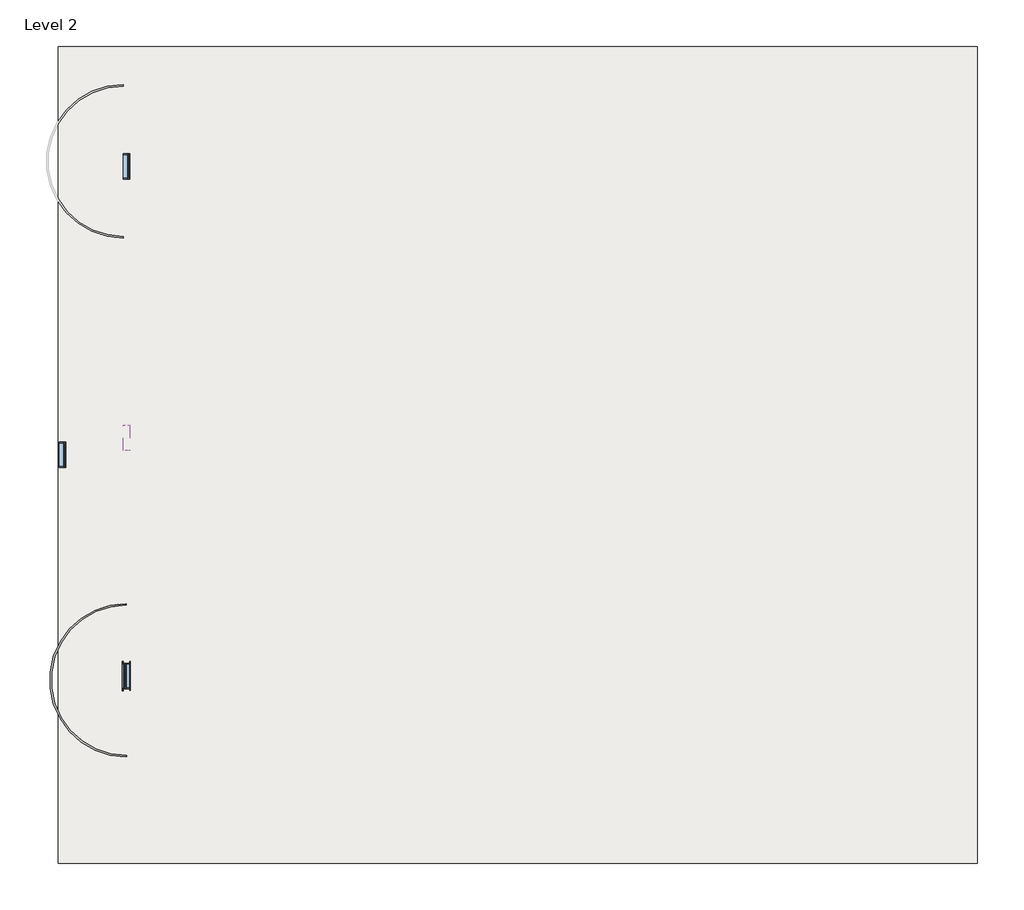
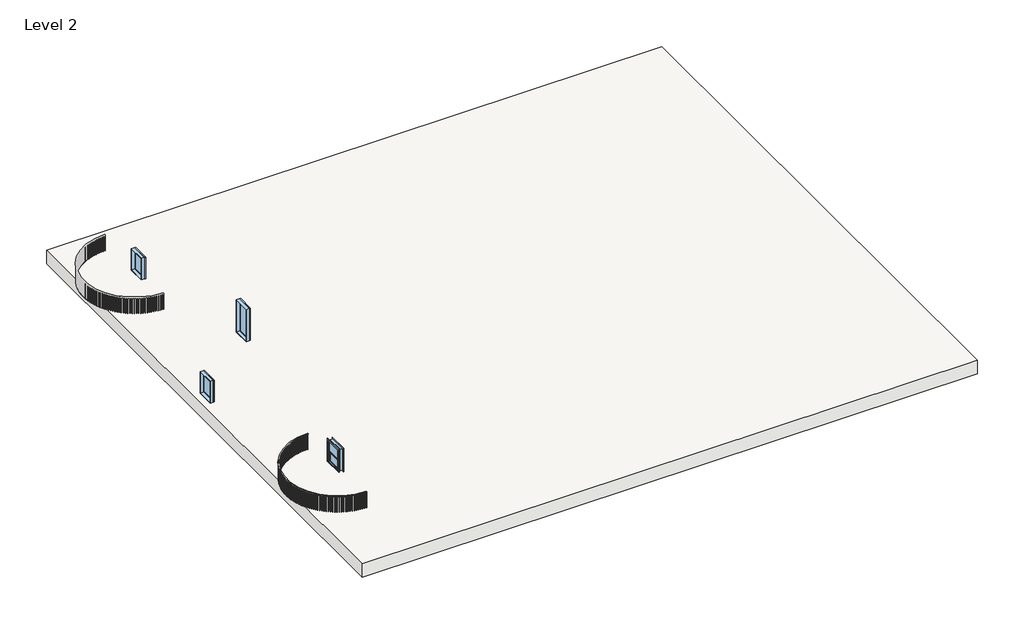
# One storey, part 1 of 2: 4 windows, 1 railing, 1 slab.
"""IFC4 building model written with IfcOpenShell, lengths in millimetres."""

from ifc_helpers import new_model, si_unit, point, frame, frame_2d, origin, place, context, project, spatial, polyline, circle_curve, trimmed, segment, composite_curve, outline, extrude, transform, mapped, element, save
from components import window_f24a59ae, window_c1f32544, window_c796fc87

model = new_model("IFC4")

# Units and contexts
model_context = context("Model", 3, world=origin())
ifc_project = project(units=[si_unit("LENGTHUNIT", "METRE", prefix="MILLI")], contexts=[model_context])

# Site, building, storey
site = spatial("IfcSite", under=ifc_project)
building = spatial("IfcBuilding", under=site)
storey = spatial("IfcBuildingStorey", under=building, Name="Level 2", Elevation=3048.0)

# Railing
placement = place(None, origin())
element("IfcRailing", 1, ObjectType="Handrail - Rectangular", at=placement, inside=storey, context=model_context, shape_type="SweptSolid", body=[
    extrude(outline(composite_curve([segment(trimmed(circle_curve(frame_2d((-15613.8723021, -8267.0443987)), 2743.2), [point((-15613.8723021, -11010.2443987))], [point((-15613.8723021, -5523.8443987))], False, "CARTESIAN"), True, "CONTINUOUS"), segment(polyline([(-15613.8723021, -5523.8443987), (-15613.8723021, -5574.6443987)]), True, "CONTINUOUS"), segment(trimmed(circle_curve(frame_2d((-15613.8723021, -8267.0443987)), 2692.4), [point((-15613.8723021, -5574.6443987))], [point((-15613.8723021, -10959.4443987))], True, "CARTESIAN"), True, "CONTINUOUS"), segment(polyline([(-15613.8723021, -10959.4443987), (-15613.8723021, -11010.2443987)]), True, "CONTINUOUS")], self_intersect=False)), frame((0.0, 0.0, 3911.6), z_axis=(0.0, 0.0, 1.0), x_axis=(1.0, 0.0, 0.0)), (0.0, 0.0, 1.0), 50.8),
    extrude(outline(polyline([(-15627.231195, -10994.3533143), (-15627.2044157, -10975.3033331), (-15608.1544345, -10975.3301124), (-15608.1812138, -10994.3800936), (-15627.231195, -10994.3533143)])), frame((0.0, 0.0, 3048.0), z_axis=(0.0, 0.0, 1.0), x_axis=(1.0, 0.0, 0.0)), (0.0, 0.0, 1.0), 863.6),
    extrude(outline(polyline([(-15729.1535895, -10991.9485449), (-15728.414846, -10972.9128742), (-15709.3791753, -10973.6516178), (-15710.1179188, -10992.6872885), (-15729.1535895, -10991.9485449)])), frame((0.0, 0.0, 3048.0), z_axis=(0.0, 0.0, 1.0), x_axis=(1.0, 0.0, 0.0)), (0.0, 0.0, 1.0), 863.6),
    extrude(outline(polyline([(-15830.914897, -10985.7361601), (-15829.4652214, -10966.7413992), (-15810.4704606, -10968.1910747), (-15811.9201361, -10987.1858356), (-15830.914897, -10985.7361601)])), frame((0.0, 0.0, 3048.0), z_axis=(0.0, 0.0, 1.0), x_axis=(1.0, 0.0, 0.0)), (0.0, 0.0, 1.0), 863.6),
    extrude(outline(polyline([(-15932.3729223, -10975.7248406), (-15930.2143405, -10956.7975316), (-15911.2870315, -10958.9561134), (-15913.4456133, -10977.8834224), (-15932.3729223, -10975.7248406)])), frame((0.0, 0.0, 3048.0), z_axis=(0.0, 0.0, 1.0), x_axis=(1.0, 0.0, 0.0)), (0.0, 0.0, 1.0), 863.6),
    extrude(outline(polyline([(-16033.3858942, -10961.9285757), (-16030.5214224, -10943.0951665), (-16011.6880132, -10945.9596384), (-16014.5524851, -10964.7930475), (-16033.3858942, -10961.9285757)])), frame((0.0, 0.0, 3048.0), z_axis=(0.0, 0.0, 1.0), x_axis=(1.0, 0.0, 0.0)), (0.0, 0.0, 1.0), 863.6),
    extrude(outline(polyline([(-16133.8126634, -10944.3666434), (-16130.2463041, -10925.6534507), (-16111.5331114, -10929.2198099), (-16115.0994706, -10947.9330026), (-16133.8126634, -10944.3666434)])), frame((0.0, 0.0, 3048.0), z_axis=(0.0, 0.0, 1.0), x_axis=(1.0, 0.0, 0.0)), (0.0, 0.0, 1.0), 863.6),
    extrude(outline(polyline([(-16233.5128994, -10923.0635838), (-16229.2496362, -10904.4967562), (-16210.6828086, -10908.7600194), (-16214.9460718, -10927.326847), (-16233.5128994, -10923.0635838)])), frame((0.0, 0.0, 3048.0), z_axis=(0.0, 0.0, 1.0), x_axis=(1.0, 0.0, 0.0)), (0.0, 0.0, 1.0), 863.6),
    extrude(outline(polyline([(-16332.3472874, -10898.0491643), (-16327.3930774, -10879.654646), (-16308.9985591, -10884.608856), (-16313.9527691, -10903.0033743), (-16332.3472874, -10898.0491643)])), frame((0.0, 0.0, 3048.0), z_axis=(0.0, 0.0, 1.0), x_axis=(1.0, 0.0, 0.0)), (0.0, 0.0, 1.0), 863.6),
    extrude(outline(polyline([(-16430.1777221, -10869.3583388), (-16424.5394881, -10851.1618331), (-16406.3429824, -10856.8000671), (-16411.9812164, -10874.9965728), (-16430.1777221, -10869.3583388)])), frame((0.0, 0.0, 3048.0), z_axis=(0.0, 0.0, 1.0), x_axis=(1.0, 0.0, 0.0)), (0.0, 0.0, 1.0), 863.6),
    extrude(outline(polyline([(-16526.8675012, -10837.0311978), (-16520.5531216, -10819.0581316), (-16502.5800554, -10825.3725111), (-16508.8944349, -10843.3455773), (-16526.8675012, -10837.0311978)])), frame((0.0, 0.0, 3048.0), z_axis=(0.0, 0.0, 1.0), x_axis=(1.0, 0.0, 0.0)), (0.0, 0.0, 1.0), 863.6),
    extrude(outline(polyline([(-16622.2815163, -10801.1129136), (-16615.2998146, -10783.3884011), (-16597.5753021, -10790.3701028), (-16604.5570038, -10808.0946153), (-16622.2815163, -10801.1129136)])), frame((0.0, 0.0, 3048.0), z_axis=(0.0, 0.0, 1.0), x_axis=(1.0, 0.0, 0.0)), (0.0, 0.0, 1.0), 863.6),
    extrude(outline(polyline([(-16716.2864416, -10761.653676), (-16708.6471735, -10744.2024845), (-16691.1959821, -10751.8417526), (-16698.8352501, -10769.292944), (-16716.2864416, -10761.653676)])), frame((0.0, 0.0, 3048.0), z_axis=(0.0, 0.0, 1.0), x_axis=(1.0, 0.0, 0.0)), (0.0, 0.0, 1.0), 863.6),
    extrude(outline(polyline([(-16808.7509204, -10718.708623), (-16800.4647607, -10701.5551378), (-16783.3112754, -10709.8412975), (-16791.5974352, -10726.9947828), (-16808.7509204, -10718.708623)])), frame((0.0, 0.0, 3048.0), z_axis=(0.0, 0.0, 1.0), x_axis=(1.0, 0.0, 0.0)), (0.0, 0.0, 1.0), 863.6),
    extrude(outline(polyline([(-16899.5457485, -10672.3377634), (-16890.6242756, -10655.5059536), (-16873.7924658, -10664.4274266), (-16882.7139387, -10681.2592364), (-16899.5457485, -10672.3377634)])), frame((0.0, 0.0, 3048.0), z_axis=(0.0, 0.0, 1.0), x_axis=(1.0, 0.0, 0.0)), (0.0, 0.0, 1.0), 863.6),
    extrude(outline(polyline([(-16988.5440547, -10622.6058931), (-16978.9997349, -10606.1192785), (-16962.5131203, -10615.6635983), (-16972.0574401, -10632.1502129), (-16988.5440547, -10622.6058931)])), frame((0.0, 0.0, 3048.0), z_axis=(0.0, 0.0, 1.0), x_axis=(1.0, 0.0, 0.0)), (0.0, 0.0, 1.0), 863.6),
    extrude(outline(polyline([(-17075.621478, -10569.5825043), (-17065.4676481, -10553.4641223), (-17049.3492661, -10563.6179523), (-17059.5030961, -10579.7363343), (-17075.621478, -10569.5825043)])), frame((0.0, 0.0, 3048.0), z_axis=(0.0, 0.0, 1.0), x_axis=(1.0, 0.0, 0.0)), (0.0, 0.0, 1.0), 863.6),
    extrude(outline(polyline([(-17160.656342, -10513.3416887), (-17149.9071902, -10497.6140622), (-17134.1795637, -10508.363214), (-17144.9287154, -10524.0908405), (-17160.656342, -10513.3416887)])), frame((0.0, 0.0, 3048.0), z_axis=(0.0, 0.0, 1.0), x_axis=(1.0, 0.0, 0.0)), (0.0, 0.0, 1.0), 863.6),
    extrude(outline(polyline([(-17243.5298239, -10453.9620338), (-17232.2003705, -10438.6471396), (-17216.8854763, -10449.976593), (-17228.2149296, -10465.2914872), (-17243.5298239, -10453.9620338)])), frame((0.0, 0.0, 3048.0), z_axis=(0.0, 0.0, 1.0), x_axis=(1.0, 0.0, 0.0)), (0.0, 0.0, 1.0), 863.6),
    extrude(outline(polyline([(-17324.1261214, -10391.5265132), (-17312.2321975, -10376.6457513), (-17297.3514357, -10388.5396752), (-17309.2453596, -10403.4204371), (-17324.1261214, -10391.5265132)])), frame((0.0, 0.0, 3048.0), z_axis=(0.0, 0.0, 1.0), x_axis=(1.0, 0.0, 0.0)), (0.0, 0.0, 1.0), 863.6),
    extrude(outline(polyline([(-17402.3326143, -10326.1223703), (-17389.8908397, -10311.6965343), (-17375.4650036, -10324.1383088), (-17387.9067782, -10338.5641449), (-17402.3326143, -10326.1223703)])), frame((0.0, 0.0, 3048.0), z_axis=(0.0, 0.0, 1.0), x_axis=(1.0, 0.0, 0.0)), (0.0, 0.0, 1.0), 863.6),
    extrude(outline(polyline([(-17478.0400213, -10257.840997), (-17465.0677814, -10243.8902446), (-17451.117029, -10256.8624845), (-17464.0892689, -10270.8132369), (-17478.0400213, -10257.840997)])), frame((0.0, 0.0, 3048.0), z_axis=(0.0, 0.0, 1.0), x_axis=(1.0, 0.0, 0.0)), (0.0, 0.0, 1.0), 863.6),
    extrude(outline(polyline([(-17551.1425537, -10186.7778056), (-17537.6579752, -10173.3216307), (-17524.2018003, -10186.8062093), (-17537.6863789, -10200.2623841), (-17551.1425537, -10186.7778056)])), frame((0.0, 0.0, 3048.0), z_axis=(0.0, 0.0, 1.0), x_axis=(1.0, 0.0, 0.0)), (0.0, 0.0, 1.0), 863.6),
    extrude(outline(polyline([(-17621.5380624, -10113.0320953), (-17607.5599877, -10100.0893009), (-17594.6171933, -10114.0673756), (-17608.595268, -10127.01017), (-17621.5380624, -10113.0320953)])), frame((0.0, 0.0, 3048.0), z_axis=(0.0, 0.0, 1.0), x_axis=(1.0, 0.0, 0.0)), (0.0, 0.0, 1.0), 863.6),
    extrude(outline(polyline([(-17689.128181, -10036.7069141), (-17674.6761422, -10024.2955856), (-17662.2648137, -10038.7476243), (-17676.7168525, -10051.1589528), (-17689.128181, -10036.7069141)])), frame((0.0, 0.0, 3048.0), z_axis=(0.0, 0.0, 1.0), x_axis=(1.0, 0.0, 0.0)), (0.0, 0.0, 1.0), 863.6),
    extrude(outline(polyline([(-17753.8184631, -9957.908914), (-17738.9126547, -9946.0463942), (-17727.0501349, -9960.9522026), (-17741.9559433, -9972.8147224), (-17753.8184631, -9957.908914)])), frame((0.0, 0.0, 3048.0), z_axis=(0.0, 0.0, 1.0), x_axis=(1.0, 0.0, 0.0)), (0.0, 0.0, 1.0), 863.6),
    extrude(outline(polyline([(-17815.5185146, -9876.7482026), (-17800.179765, -9865.4510675), (-17788.8826299, -9880.789817), (-17804.2213795, -9892.0869522), (-17815.5185146, -9876.7482026)])), frame((0.0, 0.0, 3048.0), z_axis=(0.0, 0.0, 1.0), x_axis=(1.0, 0.0, 0.0)), (0.0, 0.0, 1.0), 863.6),
    extrude(outline(polyline([(-17874.1421194, -9793.338189), (-17858.3918621, -9782.6222244), (-17847.6758976, -9798.3724817), (-17863.4261549, -9809.0884462), (-17874.1421194, -9793.338189)])), frame((0.0, 0.0, 3048.0), z_axis=(0.0, 0.0, 1.0), x_axis=(1.0, 0.0, 0.0)), (0.0, 0.0, 1.0), 863.6),
    extrude(outline(polyline([(-17929.6073606, -9707.7954251), (-17913.467604, -9697.6756051), (-17903.347784, -9713.8153616), (-17919.4875405, -9723.9351817), (-17929.6073606, -9707.7954251)])), frame((0.0, 0.0, 3048.0), z_axis=(0.0, 0.0, 1.0), x_axis=(1.0, 0.0, 0.0)), (0.0, 0.0, 1.0), 863.6),
    extrude(outline(polyline([(-17981.8367343, -9620.2394434), (-17965.3300312, -9610.7299086), (-17955.8204964, -9627.2366117), (-17972.3271995, -9636.7461465), (-17981.8367343, -9620.2394434)])), frame((0.0, 0.0, 3048.0), z_axis=(0.0, 0.0, 1.0), x_axis=(1.0, 0.0, 0.0)), (0.0, 0.0, 1.0), 863.6),
    extrude(outline(polyline([(-18030.7572585, -9530.7925891), (-18013.9066743, -9521.9066277), (-18005.0207128, -9538.7572119), (-18021.871297, -9547.6431733), (-18030.7572585, -9530.7925891)])), frame((0.0, 0.0, 3048.0), z_axis=(0.0, 0.0, 1.0), x_axis=(1.0, 0.0, 0.0)), (0.0, 0.0, 1.0), 863.6),
    extrude(outline(polyline([(-18076.3005745, -9439.5798499), (-18059.1296552, -9431.3298785), (-18050.8796837, -9448.5007978), (-18068.0506031, -9456.7507693), (-18076.3005745, -9439.5798499)])), frame((0.0, 0.0, 3048.0), z_axis=(0.0, 0.0, 1.0), x_axis=(1.0, 0.0, 0.0)), (0.0, 0.0, 1.0), 863.6),
    extrude(outline(polyline([(-18118.4030429, -9346.728681), (-18100.9357821, -9339.1262276), (-18093.3333287, -9356.5934885), (-18110.8005895, -9364.1959419), (-18118.4030429, -9346.728681)])), frame((0.0, 0.0, 3048.0), z_axis=(0.0, 0.0, 1.0), x_axis=(1.0, 0.0, 0.0)), (0.0, 0.0, 1.0), 863.6),
    extrude(outline(polyline([(-18157.0058323, -9252.3688268), (-18139.2666376, -9245.4245147), (-18132.3223254, -9263.1637094), (-18150.0615201, -9270.1080215), (-18157.0058323, -9252.3688268)])), frame((0.0, 0.0, 3048.0), z_axis=(0.0, 0.0, 1.0), x_axis=(1.0, 0.0, 0.0)), (0.0, 0.0, 1.0), 863.6),
    extrude(outline(polyline([(-18192.0550015, -9156.6321402), (-18174.0686606, -9150.3556729), (-18167.7921932, -9168.3420137), (-18185.7785341, -9174.6184811), (-18192.0550015, -9156.6321402)])), frame((0.0, 0.0, 3048.0), z_axis=(0.0, 0.0, 1.0), x_axis=(1.0, 0.0, 0.0)), (0.0, 0.0, 1.0), 863.6),
    extrude(outline(polyline([(-18223.5015748, -9059.6523978), (-18205.2932208, -9054.0525456), (-18199.6933686, -9072.2608996), (-18217.9017226, -9077.8607518), (-18223.5015748, -9059.6523978)])), frame((0.0, 0.0, 3048.0), z_axis=(0.0, 0.0, 1.0), x_axis=(1.0, 0.0, 0.0)), (0.0, 0.0, 1.0), 863.6),
    extrude(outline(polyline([(-18251.3016108, -8961.5651131), (-18232.8966869, -8956.6497009), (-18227.9812748, -8975.0546248), (-18246.3861986, -8979.970037), (-18251.3016108, -8961.5651131)])), frame((0.0, 0.0, 3048.0), z_axis=(0.0, 0.0, 1.0), x_axis=(1.0, 0.0, 0.0)), (0.0, 0.0, 1.0), 863.6),
    extrude(outline(polyline([(-18275.4162634, -8862.5073473), (-18256.8404876, -8858.2832437), (-18252.6163839, -8876.8590196), (-18271.1921598, -8881.0831232), (-18275.4162634, -8862.5073473)])), frame((0.0, 0.0, 3048.0), z_axis=(0.0, 0.0, 1.0), x_axis=(1.0, 0.0, 0.0)), (0.0, 0.0, 1.0), 863.6),
    extrude(outline(polyline([(-18295.8118362, -8762.6175179), (-18277.0911651, -8759.0906253), (-18273.5642725, -8777.8112965), (-18292.2849436, -8781.338189), (-18295.8118362, -8762.6175179)])), frame((0.0, 0.0, 3048.0), z_axis=(0.0, 0.0, 1.0), x_axis=(1.0, 0.0, 0.0)), (0.0, 0.0, 1.0), 863.6),
    extrude(outline(polyline([(-18312.4598298, -8662.0352047), (-18293.6204224, -8659.2104514), (-18290.7956691, -8678.0498587), (-18309.6350765, -8680.874612), (-18312.4598298, -8662.0352047)])), frame((0.0, 0.0, 3048.0), z_axis=(0.0, 0.0, 1.0), x_axis=(1.0, 0.0, 0.0)), (0.0, 0.0, 1.0), 863.6),
    extrude(outline(polyline([(-18325.3369811, -8560.9009553), (-18306.4051626, -8558.7822885), (-18304.2864958, -8577.714107), (-18323.2183143, -8579.8327738), (-18325.3369811, -8560.9009553)])), frame((0.0, 0.0, 3048.0), z_axis=(0.0, 0.0, 1.0), x_axis=(1.0, 0.0, 0.0)), (0.0, 0.0, 1.0), 863.6),
    extrude(outline(polyline([(-18334.4252965, -8459.3560886), (-18315.427521, -8457.9464688), (-18314.0179011, -8476.9442442), (-18333.0156766, -8478.3538641), (-18334.4252965, -8459.3560886)])), frame((0.0, 0.0, 3048.0), z_axis=(0.0, 0.0, 1.0), x_axis=(1.0, 0.0, 0.0)), (0.0, 0.0, 1.0), 863.6),
    extrude(outline(polyline([(-18339.7120764, -8357.5424973), (-18320.6748904, -8356.8438941), (-18319.9762872, -8375.8810802), (-18339.0134732, -8376.5796834), (-18339.7120764, -8357.5424973)])), frame((0.0, 0.0, 3048.0), z_axis=(0.0, 0.0, 1.0), x_axis=(1.0, 0.0, 0.0)), (0.0, 0.0, 1.0), 863.6),
    extrude(outline(polyline([(-18341.1899336, -8255.6024494), (-18322.1399383, -8255.6158391), (-18322.1533279, -8274.6658344), (-18341.2033232, -8274.6524447), (-18341.1899336, -8255.6024494)])), frame((0.0, 0.0, 3048.0), z_axis=(0.0, 0.0, 1.0), x_axis=(1.0, 0.0, 0.0)), (0.0, 0.0, 1.0), 863.6),
    extrude(outline(polyline([(-18338.8568028, -8153.6783898), (-18319.8206176, -8154.4037536), (-18320.5459814, -8173.4399388), (-18339.5821666, -8172.7145751), (-18338.8568028, -8153.6783898)])), frame((0.0, 0.0, 3048.0), z_axis=(0.0, 0.0, 1.0), x_axis=(1.0, 0.0, 0.0)), (0.0, 0.0, 1.0), 863.6),
    extrude(outline(polyline([(-18332.7159444, -8051.912741), (-18313.7201692, -8053.3490654), (-18315.1564936, -8072.3448405), (-18334.1522687, -8070.9085161), (-18332.7159444, -8051.912741)])), frame((0.0, 0.0, 3048.0), z_axis=(0.0, 0.0, 1.0), x_axis=(1.0, 0.0, 0.0)), (0.0, 0.0, 1.0), 863.6),
    extrude(outline(polyline([(-18322.775939, -7950.4477041), (-18303.8471175, -7952.592982), (-18305.9923954, -7971.5218035), (-18324.9212169, -7969.3765256), (-18322.775939, -7950.4477041)])), frame((0.0, 0.0, 3048.0), z_axis=(0.0, 0.0, 1.0), x_axis=(1.0, 0.0, 0.0)), (0.0, 0.0, 1.0), 863.6),
    extrude(outline(polyline([(-18309.0506764, -7849.4250602), (-18290.2152585, -7852.2762939), (-18293.0664923, -7871.1117118), (-18311.9019101, -7868.260478), (-18309.0506764, -7849.4250602)])), frame((0.0, 0.0, 3048.0), z_axis=(0.0, 0.0, 1.0), x_axis=(1.0, 0.0, 0.0)), (0.0, 0.0, 1.0), 863.6),
    extrude(outline(polyline([(-18291.5593353, -7748.9859721), (-18272.8436405, -7752.5391776), (-18276.396846, -7771.2548723), (-18295.1125408, -7767.7016669), (-18291.5593353, -7748.9859721)])), frame((0.0, 0.0, 3048.0), z_axis=(0.0, 0.0, 1.0), x_axis=(1.0, 0.0, 0.0)), (0.0, 0.0, 1.0), 863.6),
    extrude(outline(polyline([(-18270.3263571, -7649.2707874), (-18251.7565376, -7653.5209995), (-18256.0067497, -7672.0908191), (-18274.5765692, -7667.8406069), (-18270.3263571, -7649.2707874)])), frame((0.0, 0.0, 3048.0), z_axis=(0.0, 0.0, 1.0), x_axis=(1.0, 0.0, 0.0)), (0.0, 0.0, 1.0), 863.6),
    extrude(outline(polyline([(-18245.3814115, -7550.418842), (-18226.9834156, -7555.3601218), (-18231.9246954, -7573.7581178), (-18250.3226913, -7568.816838), (-18245.3814115, -7550.418842)])), frame((0.0, 0.0, 3048.0), z_axis=(0.0, 0.0, 1.0), x_axis=(1.0, 0.0, 0.0)), (0.0, 0.0, 1.0), 863.6),
    extrude(outline(polyline([(-18216.7593549, -7452.5682656), (-18198.5588909, -7458.1937085), (-18204.1843337, -7476.3941726), (-18222.3847978, -7470.7687297), (-18216.7593549, -7452.5682656)])), frame((0.0, 0.0, 3048.0), z_axis=(0.0, 0.0, 1.0), x_axis=(1.0, 0.0, 0.0)), (0.0, 0.0, 1.0), 863.6),
    extrude(outline(polyline([(-18184.5001822, -7355.8557887), (-18166.5226822, -7362.1575339), (-18172.8244275, -7380.1350339), (-18190.8019275, -7373.8332887), (-18184.5001822, -7355.8557887)])), frame((0.0, 0.0, 3048.0), z_axis=(0.0, 0.0, 1.0), x_axis=(1.0, 0.0, 0.0)), (0.0, 0.0, 1.0), 863.6),
    extrude(outline(polyline([(-18148.6489704, -7260.4165513), (-18130.9195551, -7267.3857933), (-18137.888797, -7285.1152086), (-18155.6182123, -7278.1459666), (-18148.6489704, -7260.4165513)])), frame((0.0, 0.0, 3048.0), z_axis=(0.0, 0.0, 1.0), x_axis=(1.0, 0.0, 0.0)), (0.0, 0.0, 1.0), 863.6),
    extrude(outline(polyline([(-18109.2558157, -7166.3839145), (-18091.7992591, -7174.0109148), (-18099.4262594, -7191.4674713), (-18116.8828159, -7183.8404711), (-18109.2558157, -7166.3839145)])), frame((0.0, 0.0, 3048.0), z_axis=(0.0, 0.0, 1.0), x_axis=(1.0, 0.0, 0.0)), (0.0, 0.0, 1.0), 863.6),
    extrude(outline(polyline([(-18066.3757637, -7073.8892738), (-18049.2164586, -7082.1633749), (-18057.4905597, -7099.32268), (-18074.6498648, -7091.0485789), (-18066.3757637, -7073.8892738)])), frame((0.0, 0.0, 3048.0), z_axis=(0.0, 0.0, 1.0), x_axis=(1.0, 0.0, 0.0)), (0.0, 0.0, 1.0), 863.6),
    extrude(outline(polyline([(-18020.0687324, -6983.0618755), (-18003.2306562, -6991.9715157), (-18012.1402963, -7008.8095919), (-18028.9783726, -6999.8999518), (-18020.0687324, -6983.0618755)])), frame((0.0, 0.0, 3048.0), z_axis=(0.0, 0.0, 1.0), x_axis=(1.0, 0.0, 0.0)), (0.0, 0.0, 1.0), 863.6),
    extrude(outline(polyline([(-17970.3994285, -6894.0286364), (-17953.9061096, -6903.5613658), (-17963.4388391, -6920.0546848), (-17979.932158, -6910.5219553), (-17970.3994285, -6894.0286364)])), frame((0.0, 0.0, 3048.0), z_axis=(0.0, 0.0, 1.0), x_axis=(1.0, 0.0, 0.0)), (0.0, 0.0, 1.0), 863.6),
    extrude(outline(polyline([(-17917.4372568, -6806.913966), (-17901.311742, -6817.0564643), (-17911.4542403, -6833.1819791), (-17927.5797552, -6823.0394808), (-17917.4372568, -6806.913966)])), frame((0.0, 0.0, 3048.0), z_axis=(0.0, 0.0, 1.0), x_axis=(1.0, 0.0, 0.0)), (0.0, 0.0, 1.0), 863.6),
    extrude(outline(polyline([(-17861.2562235, -6721.8395932), (-17845.5210456, -6732.5776878), (-17856.2591402, -6748.3128657), (-17871.9943181, -6737.5747711), (-17861.2562235, -6721.8395932)])), frame((0.0, 0.0, 3048.0), z_axis=(0.0, 0.0, 1.0), x_axis=(1.0, 0.0, 0.0)), (0.0, 0.0, 1.0), 863.6),
    extrude(outline(polyline([(-17801.9348324, -6638.9243956), (-17786.6119788, -6650.2430818), (-17797.9306651, -6665.5659354), (-17813.2535187, -6654.2472492), (-17801.9348324, -6638.9243956)])), frame((0.0, 0.0, 3048.0), z_axis=(0.0, 0.0, 1.0), x_axis=(1.0, 0.0, 0.0)), (0.0, 0.0, 1.0), 863.6),
    extrude(outline(polyline([(-17739.5559758, -6558.284234), (-17724.6668577, -6570.1676957), (-17736.5503195, -6585.0568138), (-17751.4394375, -6573.1733521), (-17739.5559758, -6558.284234)])), frame((0.0, 0.0, 3048.0), z_axis=(0.0, 0.0, 1.0), x_axis=(1.0, 0.0, 0.0)), (0.0, 0.0, 1.0), 863.6),
    extrude(outline(polyline([(-17674.206818, -6480.03179), (-17659.7722406, -6492.463422), (-17672.2038726, -6506.8979994), (-17686.63845, -6494.4663674), (-17674.206818, -6480.03179)])), frame((0.0, 0.0, 3048.0), z_axis=(0.0, 0.0, 1.0), x_axis=(1.0, 0.0, 0.0)), (0.0, 0.0, 1.0), 863.6),
    extrude(outline(polyline([(-17605.978674, -6404.2764087), (-17592.0188072, -6417.2388399), (-17604.9812384, -6431.1987066), (-17618.9411051, -6418.2362755), (-17605.978674, -6404.2764087)])), frame((0.0, 0.0, 3048.0), z_axis=(0.0, 0.0, 1.0), x_axis=(1.0, 0.0, 0.0)), (0.0, 0.0, 1.0), 863.6),
    extrude(outline(polyline([(-17534.9668816, -6331.1239463), (-17521.5012322, -6344.5990636), (-17534.9763495, -6358.064713), (-17548.4419989, -6344.5895957), (-17534.9668816, -6331.1239463)])), frame((0.0, 0.0, 3048.0), z_axis=(0.0, 0.0, 1.0), x_axis=(1.0, 0.0, 0.0)), (0.0, 0.0, 1.0), 863.6),
    extrude(outline(polyline([(-17461.2706683, -6260.6766214), (-17448.3180524, -6274.6455956), (-17462.2870265, -6287.5982116), (-17475.2396425, -6273.6292374), (-17461.2706683, -6260.6766214)])), frame((0.0, 0.0, 3048.0), z_axis=(0.0, 0.0, 1.0), x_axis=(1.0, 0.0, 0.0)), (0.0, 0.0, 1.0), 863.6),
    extrude(outline(polyline([(-17384.9930129, -6193.032873), (-17372.5715296, -6207.4761846), (-17387.0148412, -6219.897668), (-17399.4363246, -6205.4543563), (-17384.9930129, -6193.032873)])), frame((0.0, 0.0, 3048.0), z_axis=(0.0, 0.0, 1.0), x_axis=(1.0, 0.0, 0.0)), (0.0, 0.0, 1.0), 863.6),
    extrude(outline(polyline([(-17306.2405011, -6128.2872222), (-17294.3675074, -6143.1846891), (-17309.2649743, -6155.0576828), (-17321.137968, -6140.1602159), (-17306.2405011, -6128.2872222)])), frame((0.0, 0.0, 3048.0), z_axis=(0.0, 0.0, 1.0), x_axis=(1.0, 0.0, 0.0)), (0.0, 0.0, 1.0), 863.6),
    extrude(outline(polyline([(-17225.1231768, -6066.5301406), (-17213.8152633, -6081.860946), (-17229.1460687, -6093.1688594), (-17240.4539822, -6077.8380541), (-17225.1231768, -6066.5301406)])), frame((0.0, 0.0, 3048.0), z_axis=(0.0, 0.0, 1.0), x_axis=(1.0, 0.0, 0.0)), (0.0, 0.0, 1.0), 863.6),
    extrude(outline(polyline([(-17141.7543884, -6007.847924), (-17131.0273562, -6023.5906455), (-17146.7700777, -6034.3176777), (-17157.4971099, -6018.5749562), (-17141.7543884, -6007.847924)])), frame((0.0, 0.0, 3048.0), z_axis=(0.0, 0.0, 1.0), x_axis=(1.0, 0.0, 0.0)), (0.0, 0.0, 1.0), 863.6),
    extrude(outline(polyline([(-17056.2506305, -5952.3225712), (-17046.1194688, -5968.4552108), (-17062.2521085, -5978.5863725), (-17072.3832702, -5962.4537328), (-17056.2506305, -5952.3225712)])), frame((0.0, 0.0, 3048.0), z_axis=(0.0, 0.0, 1.0), x_axis=(1.0, 0.0, 0.0)), (0.0, 0.0, 1.0), 863.6),
    extrude(outline(polyline([(-16968.7313808, -5900.03167), (-16959.2102463, -5916.5316851), (-16975.7102614, -5926.0528195), (-16985.2313959, -5909.5528044), (-16968.7313808, -5900.03167)])), frame((0.0, 0.0, 3048.0), z_axis=(0.0, 0.0, 1.0), x_axis=(1.0, 0.0, 0.0)), (0.0, 0.0, 1.0), 863.6),
    extrude(outline(polyline([(-16879.3189333, -5851.0482885), (-16870.4211303, -5867.8926229), (-16887.2654647, -5876.7904259), (-16896.1632677, -5859.9460915), (-16879.3189333, -5851.0482885)])), frame((0.0, 0.0, 3048.0), z_axis=(0.0, 0.0, 1.0), x_axis=(1.0, 0.0, 0.0)), (0.0, 0.0, 1.0), 863.6),
    extrude(outline(polyline([(-16788.1382277, -5805.4408731), (-16779.8761894, -5822.6059896), (-16797.0413058, -5830.8680279), (-16805.3033441, -5813.7029114), (-16788.1382277, -5805.4408731)])), frame((0.0, 0.0, 3048.0), z_axis=(0.0, 0.0, 1.0), x_axis=(1.0, 0.0, 0.0)), (0.0, 0.0, 1.0), 863.6),
    extrude(outline(polyline([(-16695.3166742, -5763.2731529), (-16687.7019455, -5780.7350659), (-16705.1638585, -5788.3497946), (-16712.7785872, -5770.8878816), (-16695.3166742, -5763.2731529)])), frame((0.0, 0.0, 3048.0), z_axis=(0.0, 0.0, 1.0), x_axis=(1.0, 0.0, 0.0)), (0.0, 0.0, 1.0), 863.6),
    extrude(outline(polyline([(-16600.983976, -5724.6040505), (-16594.0271973, -5742.3383598), (-16611.7615066, -5749.2951386), (-16618.7182854, -5731.5608292), (-16600.983976, -5724.6040505)])), frame((0.0, 0.0, 3048.0), z_axis=(0.0, 0.0, 1.0), x_axis=(1.0, 0.0, 0.0)), (0.0, 0.0, 1.0), 863.6),
    extrude(outline(polyline([(-16505.271948, -5689.4875996), (-16498.9828402, -5707.4695245), (-16516.9647651, -5713.7586324), (-16523.2538729, -5695.7767075), (-16505.271948, -5689.4875996)])), frame((0.0, 0.0, 3048.0), z_axis=(0.0, 0.0, 1.0), x_axis=(1.0, 0.0, 0.0)), (0.0, 0.0, 1.0), 863.6),
    extrude(outline(polyline([(-16408.3143324, -5657.97287), (-16402.7016834, -5676.1772836), (-16420.906097, -5681.7899325), (-16426.5187459, -5663.5855189), (-16408.3143324, -5657.97287)])), frame((0.0, 0.0, 3048.0), z_axis=(0.0, 0.0, 1.0), x_axis=(1.0, 0.0, 0.0)), (0.0, 0.0, 1.0), 863.6),
    extrude(outline(polyline([(-16310.2466117, -5630.1038984), (-16305.3182645, -5648.5053628), (-16323.7197289, -5653.43371), (-16328.6480761, -5635.0322456), (-16310.2466117, -5630.1038984)])), frame((0.0, 0.0, 3048.0), z_axis=(0.0, 0.0, 1.0), x_axis=(1.0, 0.0, 0.0)), (0.0, 0.0, 1.0), 863.6),
    extrude(outline(polyline([(-16211.2058198, -5605.9196271), (-16206.9686609, -5624.4924294), (-16225.5414632, -5628.7295883), (-16229.7786221, -5610.1567861), (-16211.2058198, -5605.9196271)])), frame((0.0, 0.0, 3048.0), z_axis=(0.0, 0.0, 1.0), x_axis=(1.0, 0.0, 0.0)), (0.0, 0.0, 1.0), 863.6),
    extrude(outline(polyline([(-16111.3303505, -5585.4538499), (-16107.7903006, -5604.1720375), (-16126.5084882, -5607.7120874), (-16130.048538, -5588.9938998), (-16111.3303505, -5585.4538499)])), frame((0.0, 0.0, 3048.0), z_axis=(0.0, 0.0, 1.0), x_axis=(1.0, 0.0, 0.0)), (0.0, 0.0, 1.0), 863.6),
    extrude(outline(polyline([(-16010.7597634, -5568.7351643), (-16007.9217692, -5587.5725816), (-16026.7591865, -5590.4105758), (-16029.5971807, -5571.5731585), (-16010.7597634, -5568.7351643)])), frame((0.0, 0.0, 3048.0), z_axis=(0.0, 0.0, 1.0), x_axis=(1.0, 0.0, 0.0)), (0.0, 0.0, 1.0), 863.6),
    extrude(outline(polyline([(-15909.63459, -5555.7869321), (-15907.5026171, -5574.7172567), (-15926.4329418, -5576.8492296), (-15928.5649146, -5557.918905), (-15909.63459, -5555.7869321)])), frame((0.0, 0.0, 3048.0), z_axis=(0.0, 0.0, 1.0), x_axis=(1.0, 0.0, 0.0)), (0.0, 0.0, 1.0), 863.6),
    extrude(outline(polyline([(-15808.0961363, -5546.6272462), (-15806.6731638, -5565.6240262), (-15825.6699438, -5567.0469987), (-15827.0929163, -5548.0502187), (-15808.0961363, -5546.6272462)])), frame((0.0, 0.0, 3048.0), z_axis=(0.0, 0.0, 1.0), x_axis=(1.0, 0.0, 0.0)), (0.0, 0.0, 1.0), 863.6),
    extrude(outline(polyline([(-15706.286286, -5541.268906), (-15705.5743024, -5560.3055963), (-15724.6109927, -5561.01758), (-15725.3229764, -5541.9808896), (-15706.286286, -5541.268906)])), frame((0.0, 0.0, 3048.0), z_axis=(0.0, 0.0, 1.0), x_axis=(1.0, 0.0, 0.0)), (0.0, 0.0, 1.0), 863.6),
    extrude(outline(polyline([(-15632.955606, -10994.3192673), (-15632.8888422, -10975.2693843), (-15613.8389591, -10975.3361482), (-15613.905723, -10994.3860312), (-15632.955606, -10994.3192673)])), frame((0.0, 0.0, 3048.0), z_axis=(0.0, 0.0, 1.0), x_axis=(1.0, 0.0, 0.0)), (0.0, 0.0, 1.0), 863.6),
    extrude(outline(polyline([(-15613.905723, -5539.7027662), (-15613.8389591, -5558.7526493), (-15632.8888422, -5558.8194131), (-15632.955606, -5539.7695301), (-15613.905723, -5539.7027662)])), frame((0.0, 0.0, 3048.0), z_axis=(0.0, 0.0, 1.0), x_axis=(1.0, 0.0, 0.0)), (0.0, 0.0, 1.0), 863.6),
])

# Slab
element("IfcSlab", 2, ObjectType="Generic - 12\"", at=placement, inside=storey, context=model_context, shape_type="SweptSolid", body=[
    extrude(outline(polyline([(14866.1276979, 14440.5556013), (14866.1276979, -14820.2443987), (-18052.2723021, -14820.2443987), (-18052.2723021, 14440.5556013), (14866.1276979, 14440.5556013)])), frame((0.0, 0.0, 2286.0), z_axis=(0.0, 0.0, 1.0), x_axis=(1.0, 0.0, 0.0)), (0.0, 0.0, 1.0), 762.0),
])

# Windows
window_shape = window_f24a59ae(model_context)
element("IfcWindow", 3, ObjectType="Double Hung with Trim : 36\" x 48\"", at=placement, inside=storey, context=model_context, shape_type="MappedRepresentation", body=[
    mapped(window_shape, transform((-15613.8723021, -8114.6443987, 2757.7089798), x_axis=(0.0, 1.0, 0.0), y_axis=(-1.0, 0.0, 0.0), z_axis=(0.0, 0.0, 1.0))),
])
window_2_shape = window_c1f32544(model_context)
element("IfcWindow", 4, ObjectType="Fixed : 36\" x 48\"", at=placement, inside=storey, context=model_context, shape_type="MappedRepresentation", body=[
    mapped(window_2_shape, transform((-15613.8723021, 10109.8556013, 2518.9653391), x_axis=(0.0, -1.0, 0.0), y_axis=(1.0, 0.0, 0.0), z_axis=(0.0, 0.0, 1.0))),
])
element("IfcWindow", 5, ObjectType="Fixed : 36\" x 48\"", at=placement, inside=storey, context=model_context, shape_type="MappedRepresentation", body=[
    mapped(window_2_shape, transform((-17899.8723021, -227.9443987, 2627.364574), x_axis=(0.0, -1.0, 0.0), y_axis=(1.0, 0.0, 0.0), z_axis=(0.0, 0.0, 1.0))),
])
window_3_shape = window_c796fc87(model_context)
element("IfcWindow", 6, ObjectType="Fixed : 36\" x 72\"", at=placement, inside=storey, context=model_context, shape_type="MappedRepresentation", body=[
    mapped(window_3_shape, transform((-15613.8723021, 381.6556013, 5529.0452052), x_axis=(0.0, -1.0, 0.0), y_axis=(1.0, 0.0, 0.0), z_axis=(0.0, 0.0, 1.0))),
])

save(model, "model.ifc")

# Revit data of these elements
# Type "Handrail - Rectangular"
#   Assembly Code = "C2010400"
#   built-in parameter 1008612 = 0.0416667 (stored number, unit not read)
#   built-in parameter 1008611 = 0.0416667 (stored number, unit not read)
#   built-in parameter 1008609 = 0.333333 (stored number, unit not read)
#   built-in parameter 1008604 = 0.166667 (stored number, unit not read)
#   built-in parameter 1008603 = 0.166667 (stored number, unit not read)
#   Railing Height = 3' - 0"
#   built-in parameter 1008630 = 2
#   built-in parameter 1008610 = 2
#   built-in parameter 1008618 = Baluster - Square : 3/4"
# Type "Generic - 12\""
#   Assembly Code = "B1010"
#   Function = 0
#   Layers, outside or top first: 2' - 6" no material (function 1)
# Type "Double Hung with Trim : 36\" x 48\""
#   Type Mark = "10"
#   Construction Type Id = "GSP4R"
#   Assembly Code = "B2020100"
#   Analytic Construction = "1/8 in Pilkington single glazing"
#   Visual Light Transmittance = 0.9
#   Solar Heat Gain Coefficient = 0.78
#   Heat Transfer Coefficient (U) = 0.6496 BTU/(h·ft²·°F)
#   Height = 4' - 0"
#   Default Sill Height = 3' - 0"
#   Trim Projection - Ext. = 0' - 0 1/2"
#   Trim Projection - Int. = 0' - 0 3/4"
#   Trim Width - Exterior = 0' - 3 1/2"
#   Trim Width - Interior = 0' - 3 1/2"
#   Width = 3' - 0"
#   Window Inset = 0' - 0 3/4"
#   Define Thermal Properties by = 1
#   Glass Pane Material = Glass
#   Sash Material = Sash
#   Trim Exterior Material = Trim
#   Trim Interior Material = Trim
#   Wall Closure = (empty or 0)
# Type "Fixed : 36\" x 48\""
#   Type Mark = "1"
#   Construction Type Id = "GSP4R"
#   Assembly Code = "B2020100"
#   Analytic Construction = "1/8 in Pilkington single glazing"
#   Visual Light Transmittance = 0.9
#   Solar Heat Gain Coefficient = 0.78
#   Heat Transfer Coefficient (U) = 0.6496 BTU/(h·ft²·°F)
#   Height = 4' - 0"
#   Default Sill Height = 3' - 0"
#   Width = 3' - 0"
#   Window Inset = 0' - 0 3/4"
#   Define Thermal Properties by = 1
#   Glass Pane Material = Glass
#   Sash Material = Sash
#   Wall Closure = (empty or 0)
# Type "Fixed : 36\" x 72\""
#   Type Mark = "9"
#   Construction Type Id = "GSP4R"
#   Assembly Code = "B2020100"
#   Analytic Construction = "1/8 in Pilkington single glazing"
#   Visual Light Transmittance = 0.9
#   Solar Heat Gain Coefficient = 0.78
#   Heat Transfer Coefficient (U) = 0.6496 BTU/(h·ft²·°F)
#   Height = 6' - 0"
#   Default Sill Height = 1' - 0"
#   Width = 3' - 0"
#   Window Inset = 0' - 0 3/4"
#   Define Thermal Properties by = 1
#   Glass Pane Material = Glass
#   Sash Material = Sash
#   Wall Closure = (empty or 0)
# Element 1 (IfcRailing, "Handrail - Rectangular")
#   Phase Created = New Construction
# Element 2 (IfcSlab, "Generic - 12\"")
#   Height Offset From Level = 0' - 0"
#   Phase Created = New Construction
#   Materials on its faces: "Default Floor"
# Element 3 (IfcWindow, "Double Hung with Trim : 36\" x 48\"")
#   Mark = "6"
#   Phase Created = New Construction
#   Materials on its faces: "Sash", "Trim", "Glass"
# Element 4 (IfcWindow, "Fixed : 36\" x 48\"")
#   Mark = "5"
#   Phase Created = New Construction
#   Materials on its faces: "Sash", "Glass"
# Element 5 (IfcWindow, "Fixed : 36\" x 48\"")
#   Mark = "23"
#   Phase Created = New Construction
#   Materials on its faces: "Sash", "Glass"
# Element 6 (IfcWindow, "Fixed : 36\" x 72\"")
#   Mark = "16"
#   Phase Created = New Construction
#   Materials on its faces: "Sash", "Glass"
# Materials
#   "Glass": class "Glass", colour RGB 0 128 192, transparency 0.75, Description = "Soda Lime Glass", Cost = 0
#   "Sash": class "Wood", colour RGB 224 178 126, transparency 0
#   "Trim": class "Wood", colour RGB 224 178 126, transparency 0
#   "Default Floor": colour RGB 128 128 128, transparency 0
